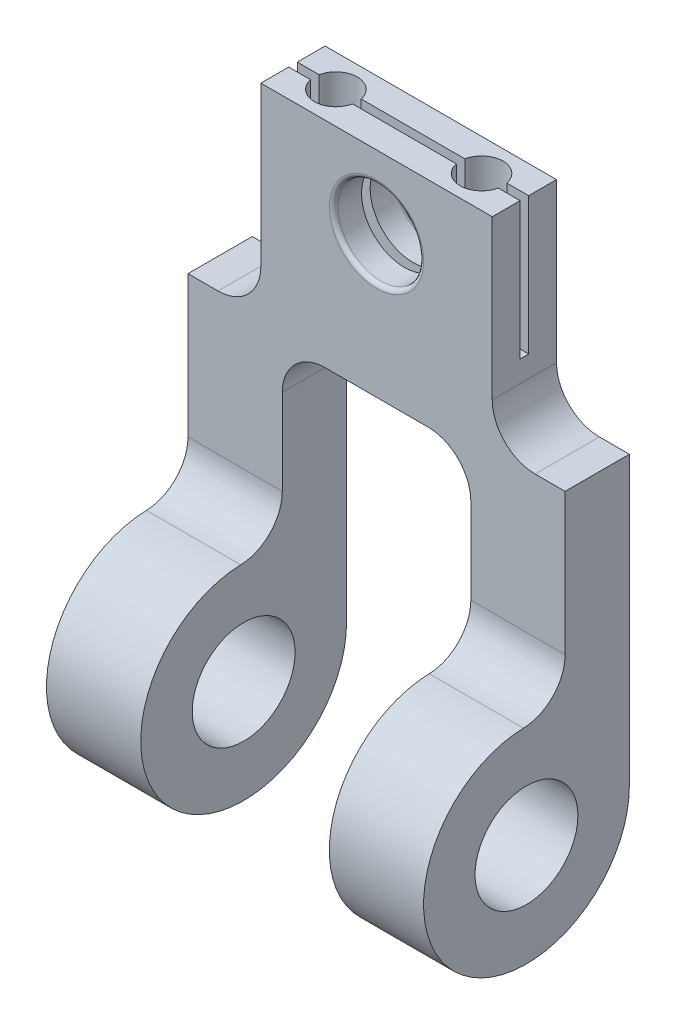
ISO-10303-21;
HEADER;
FILE_DESCRIPTION(('STEP AP214'),'2;1');
FILE_NAME('part.step','',(''),(''),'','','');
FILE_SCHEMA(('AUTOMOTIVE_DESIGN { 1 0 10303 214 1 1 1 1 }'));
ENDSEC;
DATA;
#1=APPLICATION_CONTEXT('core data for automotive mechanical design processes');
#2=APPLICATION_PROTOCOL_DEFINITION('international standard','automotive_design',2000,#1);
#3=PRODUCT_CONTEXT('',#1,'mechanical');
#4=PRODUCT('Part','Part','',(#3));
#5=PRODUCT_RELATED_PRODUCT_CATEGORY('part','',(#4));
#6=PRODUCT_DEFINITION_FORMATION('','',#4);
#7=PRODUCT_DEFINITION_CONTEXT('part definition',#1,'design');
#8=PRODUCT_DEFINITION('design','',#6,#7);
#9=PRODUCT_DEFINITION_SHAPE('','',#8);
#10=(LENGTH_UNIT() NAMED_UNIT(*) SI_UNIT(.MILLI.,.METRE.));
#11=(NAMED_UNIT(*) PLANE_ANGLE_UNIT() SI_UNIT($,.RADIAN.));
#12=(NAMED_UNIT(*) SI_UNIT($,.STERADIAN.) SOLID_ANGLE_UNIT());
#13=UNCERTAINTY_MEASURE_WITH_UNIT(LENGTH_MEASURE(1.E-05),#10,'distance_accuracy_value','');
#14=(GEOMETRIC_REPRESENTATION_CONTEXT(3) GLOBAL_UNCERTAINTY_ASSIGNED_CONTEXT((#13)) GLOBAL_UNIT_ASSIGNED_CONTEXT((#10,
#11,#12)) REPRESENTATION_CONTEXT('',''));
#15=CARTESIAN_POINT('',(0.,0.,0.));
#16=DIRECTION('',(0.,0.,1.));
#17=DIRECTION('',(1.,0.,0.));
#18=AXIS2_PLACEMENT_3D('',#15,#16,#17);
#19=CARTESIAN_POINT('',(44.,114.,-24.01));
#20=DIRECTION('',(0.,-1.,0.));
#21=DIRECTION('',(0.,0.,-1.));
#22=AXIS2_PLACEMENT_3D('',#19,#20,#21);
#23=PLANE('',#22);
#24=CARTESIAN_POINT('',(-17.,114.,-16.51));
#25=DIRECTION('',(0.,1.,0.));
#26=DIRECTION('',(0.,0.,1.));
#27=AXIS2_PLACEMENT_3D('',#24,#25,#26);
#28=CIRCLE('',#27,5.);
#29=CARTESIAN_POINT('',(-21.8989794855664,114.,-15.51));
#30=VERTEX_POINT('',#29);
#31=CARTESIAN_POINT('',(-12.1010205144336,114.,-15.51));
#32=VERTEX_POINT('',#31);
#33=EDGE_CURVE('E499',#30,#32,#28,.T.);
#34=ORIENTED_EDGE('',*,*,#33,.F.);
#35=DIRECTION('',(1.,0.,0.));
#36=VECTOR('',#35,1.);
#37=CARTESIAN_POINT('',(-44.,114.,-15.51));
#38=LINE('',#37,#36);
#39=CARTESIAN_POINT('',(-27.,114.,-15.51));
#40=VERTEX_POINT('',#39);
#41=EDGE_CURVE('E263',#40,#30,#38,.T.);
#42=ORIENTED_EDGE('',*,*,#41,.F.);
#43=DIRECTION('',(0.,0.,1.));
#44=VECTOR('',#43,1.);
#45=CARTESIAN_POINT('',(-27.,114.,-24.01));
#46=LINE('',#45,#44);
#47=CARTESIAN_POINT('',(-27.,114.,-9.01));
#48=VERTEX_POINT('',#47);
#49=EDGE_CURVE('E296',#40,#48,#46,.T.);
#50=ORIENTED_EDGE('',*,*,#49,.T.);
#51=DIRECTION('',(-1.,0.,0.));
#52=VECTOR('',#51,1.);
#53=CARTESIAN_POINT('',(44.,114.,-9.01));
#54=LINE('',#53,#52);
#55=CARTESIAN_POINT('',(27.,114.,-9.01));
#56=VERTEX_POINT('',#55);
#57=EDGE_CURVE('E338',#56,#48,#54,.T.);
#58=ORIENTED_EDGE('',*,*,#57,.F.);
#59=DIRECTION('',(0.,0.,1.));
#60=VECTOR('',#59,1.);
#61=CARTESIAN_POINT('',(27.,114.,-24.01));
#62=LINE('',#61,#60);
#63=CARTESIAN_POINT('',(27.,114.,-15.51));
#64=VERTEX_POINT('',#63);
#65=EDGE_CURVE('E256',#64,#56,#62,.T.);
#66=ORIENTED_EDGE('',*,*,#65,.F.);
#67=CARTESIAN_POINT('',(21.8989794855664,114.,-15.51));
#68=VERTEX_POINT('',#67);
#69=EDGE_CURVE('E252',#68,#64,#38,.T.);
#70=ORIENTED_EDGE('',*,*,#69,.F.);
#71=CARTESIAN_POINT('',(17.,114.,-16.51));
#72=DIRECTION('',(0.,1.,0.));
#73=DIRECTION('',(0.,0.,1.));
#74=AXIS2_PLACEMENT_3D('',#71,#72,#73);
#75=CIRCLE('',#74,5.);
#76=CARTESIAN_POINT('',(12.1010205144336,114.,-15.51));
#77=VERTEX_POINT('',#76);
#78=EDGE_CURVE('E234',#77,#68,#75,.T.);
#79=ORIENTED_EDGE('',*,*,#78,.F.);
#80=EDGE_CURVE('E258',#32,#77,#38,.T.);
#81=ORIENTED_EDGE('',*,*,#80,.F.);
#82=EDGE_LOOP('',(#34,#42,#50,#58,#66,#70,#79,#81));
#83=FACE_BOUND('',#82,.T.);
#84=ADVANCED_FACE('F39',(#83),#23,.F.);
#85=CARTESIAN_POINT('',(-12.1010205144336,114.,-17.51));
#86=VERTEX_POINT('',#85);
#87=CARTESIAN_POINT('',(-21.8989794855664,114.,-17.51));
#88=VERTEX_POINT('',#87);
#89=EDGE_CURVE('E505',#86,#88,#28,.T.);
#90=ORIENTED_EDGE('',*,*,#89,.F.);
#91=DIRECTION('',(1.,0.,0.));
#92=VECTOR('',#91,1.);
#93=CARTESIAN_POINT('',(-44.,114.,-17.51));
#94=LINE('',#93,#92);
#95=CARTESIAN_POINT('',(12.1010205144336,114.,-17.51));
#96=VERTEX_POINT('',#95);
#97=EDGE_CURVE('E261',#86,#96,#94,.T.);
#98=ORIENTED_EDGE('',*,*,#97,.T.);
#99=CARTESIAN_POINT('',(21.8989794855664,114.,-17.51));
#100=VERTEX_POINT('',#99);
#101=EDGE_CURVE('E244',#100,#96,#75,.T.);
#102=ORIENTED_EDGE('',*,*,#101,.F.);
#103=CARTESIAN_POINT('',(27.,114.,-17.51));
#104=VERTEX_POINT('',#103);
#105=EDGE_CURVE('E270',#100,#104,#94,.T.);
#106=ORIENTED_EDGE('',*,*,#105,.T.);
#107=CARTESIAN_POINT('',(27.,114.,-24.01));
#108=VERTEX_POINT('',#107);
#109=EDGE_CURVE('E304',#108,#104,#62,.T.);
#110=ORIENTED_EDGE('',*,*,#109,.F.);
#111=DIRECTION('',(-1.,0.,0.));
#112=VECTOR('',#111,1.);
#113=CARTESIAN_POINT('',(44.,114.,-24.01));
#114=LINE('',#113,#112);
#115=CARTESIAN_POINT('',(-27.,114.,-24.01));
#116=VERTEX_POINT('',#115);
#117=EDGE_CURVE('E347',#108,#116,#114,.T.);
#118=ORIENTED_EDGE('',*,*,#117,.T.);
#119=CARTESIAN_POINT('',(-27.,114.,-17.51));
#120=VERTEX_POINT('',#119);
#121=EDGE_CURVE('E295',#116,#120,#46,.T.);
#122=ORIENTED_EDGE('',*,*,#121,.T.);
#123=EDGE_CURVE('E262',#120,#88,#94,.T.);
#124=ORIENTED_EDGE('',*,*,#123,.T.);
#125=EDGE_LOOP('',(#90,#98,#102,#106,#110,#118,#122,#124));
#126=FACE_BOUND('',#125,.T.);
#127=ADVANCED_FACE('F512',(#126),#23,.F.);
#128=CARTESIAN_POINT('',(-44.,114.,-15.51));
#129=DIRECTION('',(0.,0.,1.));
#130=DIRECTION('',(0.,-1.,0.));
#131=AXIS2_PLACEMENT_3D('',#128,#129,#130);
#132=PLANE('',#131);
#133=CARTESIAN_POINT('',(0.,97.,-15.51));
#134=DIRECTION('',(0.,0.,1.));
#135=DIRECTION('',(0.,-1.,0.));
#136=AXIS2_PLACEMENT_3D('',#133,#134,#135);
#137=CIRCLE('',#136,10.);
#138=CARTESIAN_POINT('',(0.,87.,-15.51));
#139=VERTEX_POINT('',#138);
#140=EDGE_CURVE('E447',#139,#139,#137,.T.);
#141=ORIENTED_EDGE('',*,*,#140,.T.);
#142=EDGE_LOOP('',(#141));
#143=FACE_BOUND('',#142,.T.);
#144=DIRECTION('',(1.,0.,0.));
#145=VECTOR('',#144,1.);
#146=CARTESIAN_POINT('',(-44.,82.,-15.51));
#147=LINE('',#146,#145);
#148=CARTESIAN_POINT('',(-12.1010205144336,82.,-15.51));
#149=VERTEX_POINT('',#148);
#150=CARTESIAN_POINT('',(12.1010205144336,82.,-15.51));
#151=VERTEX_POINT('',#150);
#152=EDGE_CURVE('E476',#149,#151,#147,.T.);
#153=ORIENTED_EDGE('',*,*,#152,.F.);
#154=DIRECTION('',(0.,1.,0.));
#155=VECTOR('',#154,1.);
#156=CARTESIAN_POINT('',(-12.1010205144336,65.,-15.51));
#157=LINE('',#156,#155);
#158=EDGE_CURVE('E450',#149,#32,#157,.T.);
#159=ORIENTED_EDGE('',*,*,#158,.T.);
#160=ORIENTED_EDGE('',*,*,#80,.T.);
#161=DIRECTION('',(0.,1.,0.));
#162=VECTOR('',#161,1.);
#163=CARTESIAN_POINT('',(12.1010205144336,65.,-15.51));
#164=LINE('',#163,#162);
#165=EDGE_CURVE('E239',#77,#151,#164,.F.);
#166=ORIENTED_EDGE('',*,*,#165,.T.);
#167=EDGE_LOOP('',(#153,#159,#160,#166));
#168=FACE_BOUND('',#167,.T.);
#169=ADVANCED_FACE('F519',(#143,#168),#132,.F.);
#170=CARTESIAN_POINT('',(21.8989794855664,82.,-15.51));
#171=VERTEX_POINT('',#170);
#172=CARTESIAN_POINT('',(27.,82.,-15.51));
#173=VERTEX_POINT('',#172);
#174=EDGE_CURVE('E254',#171,#173,#147,.T.);
#175=ORIENTED_EDGE('',*,*,#174,.F.);
#176=DIRECTION('',(0.,1.,0.));
#177=VECTOR('',#176,1.);
#178=CARTESIAN_POINT('',(21.8989794855664,65.,-15.51));
#179=LINE('',#178,#177);
#180=EDGE_CURVE('E240',#171,#68,#179,.T.);
#181=ORIENTED_EDGE('',*,*,#180,.T.);
#182=ORIENTED_EDGE('',*,*,#69,.T.);
#183=DIRECTION('',(0.,1.,0.));
#184=VECTOR('',#183,1.);
#185=CARTESIAN_POINT('',(27.,114.,-15.51));
#186=LINE('',#185,#184);
#187=EDGE_CURVE('E278',#173,#64,#186,.T.);
#188=ORIENTED_EDGE('',*,*,#187,.F.);
#189=EDGE_LOOP('',(#175,#181,#182,#188));
#190=FACE_BOUND('',#189,.T.);
#191=ADVANCED_FACE('F248',(#190),#132,.F.);
#192=CARTESIAN_POINT('',(-44.,114.,-17.51));
#193=DIRECTION('',(0.,0.,-1.));
#194=DIRECTION('',(0.,1.,0.));
#195=AXIS2_PLACEMENT_3D('',#192,#193,#194);
#196=PLANE('',#195);
#197=DIRECTION('',(1.,0.,0.));
#198=VECTOR('',#197,1.);
#199=CARTESIAN_POINT('',(-44.,82.,-17.51));
#200=LINE('',#199,#198);
#201=CARTESIAN_POINT('',(-27.,82.,-17.51));
#202=VERTEX_POINT('',#201);
#203=CARTESIAN_POINT('',(-21.8989794855664,82.,-17.51));
#204=VERTEX_POINT('',#203);
#205=EDGE_CURVE('E468',#202,#204,#200,.T.);
#206=ORIENTED_EDGE('',*,*,#205,.T.);
#207=DIRECTION('',(0.,1.,0.));
#208=VECTOR('',#207,1.);
#209=CARTESIAN_POINT('',(-21.8989794855664,65.,-17.51));
#210=LINE('',#209,#208);
#211=EDGE_CURVE('E65',#204,#88,#210,.T.);
#212=ORIENTED_EDGE('',*,*,#211,.T.);
#213=ORIENTED_EDGE('',*,*,#123,.F.);
#214=DIRECTION('',(0.,1.,0.));
#215=VECTOR('',#214,1.);
#216=CARTESIAN_POINT('',(-27.,114.,-17.51));
#217=LINE('',#216,#215);
#218=EDGE_CURVE('E436',#202,#120,#217,.T.);
#219=ORIENTED_EDGE('',*,*,#218,.F.);
#220=EDGE_LOOP('',(#206,#212,#213,#219));
#221=FACE_BOUND('',#220,.T.);
#222=ADVANCED_FACE('F471',(#221),#196,.F.);
#223=CARTESIAN_POINT('',(0.,97.,-17.51));
#224=DIRECTION('',(0.,0.,-1.));
#225=DIRECTION('',(0.,1.,0.));
#226=AXIS2_PLACEMENT_3D('',#223,#224,#225);
#227=CIRCLE('',#226,10.);
#228=CARTESIAN_POINT('',(0.,107.,-17.51));
#229=VERTEX_POINT('',#228);
#230=EDGE_CURVE('E442',#229,#229,#227,.T.);
#231=ORIENTED_EDGE('',*,*,#230,.T.);
#232=EDGE_LOOP('',(#231));
#233=FACE_BOUND('',#232,.T.);
#234=ORIENTED_EDGE('',*,*,#97,.F.);
#235=DIRECTION('',(0.,1.,0.));
#236=VECTOR('',#235,1.);
#237=CARTESIAN_POINT('',(-12.1010205144336,65.,-17.51));
#238=LINE('',#237,#236);
#239=CARTESIAN_POINT('',(-12.1010205144336,82.,-17.51));
#240=VERTEX_POINT('',#239);
#241=EDGE_CURVE('E487',#86,#240,#238,.F.);
#242=ORIENTED_EDGE('',*,*,#241,.T.);
#243=CARTESIAN_POINT('',(12.1010205144336,82.,-17.51));
#244=VERTEX_POINT('',#243);
#245=EDGE_CURVE('E473',#240,#244,#200,.T.);
#246=ORIENTED_EDGE('',*,*,#245,.T.);
#247=DIRECTION('',(0.,1.,0.));
#248=VECTOR('',#247,1.);
#249=CARTESIAN_POINT('',(12.1010205144336,65.,-17.51));
#250=LINE('',#249,#248);
#251=EDGE_CURVE('E53',#244,#96,#250,.T.);
#252=ORIENTED_EDGE('',*,*,#251,.T.);
#253=EDGE_LOOP('',(#234,#242,#246,#252));
#254=FACE_BOUND('',#253,.T.);
#255=ADVANCED_FACE('F511',(#233,#254),#196,.F.);
#256=CARTESIAN_POINT('',(-44.,82.,-15.51));
#257=DIRECTION('',(0.,-1.,0.));
#258=DIRECTION('',(0.,0.,-1.));
#259=AXIS2_PLACEMENT_3D('',#256,#257,#258);
#260=PLANE('',#259);
#261=ORIENTED_EDGE('',*,*,#245,.F.);
#262=CARTESIAN_POINT('',(-17.,82.,-16.51));
#263=DIRECTION('',(0.,-1.,0.));
#264=DIRECTION('',(0.,0.,-1.));
#265=AXIS2_PLACEMENT_3D('',#262,#263,#264);
#266=CIRCLE('',#265,5.);
#267=EDGE_CURVE('E11',#240,#149,#266,.T.);
#268=ORIENTED_EDGE('',*,*,#267,.T.);
#269=ORIENTED_EDGE('',*,*,#152,.T.);
#270=CARTESIAN_POINT('',(17.,82.,-16.51));
#271=DIRECTION('',(0.,-1.,0.));
#272=DIRECTION('',(0.,0.,-1.));
#273=AXIS2_PLACEMENT_3D('',#270,#271,#272);
#274=CIRCLE('',#273,5.);
#275=EDGE_CURVE('E458',#151,#244,#274,.T.);
#276=ORIENTED_EDGE('',*,*,#275,.T.);
#277=EDGE_LOOP('',(#261,#268,#269,#276));
#278=FACE_BOUND('',#277,.T.);
#279=ADVANCED_FACE('F513',(#278),#260,.F.);
#280=CARTESIAN_POINT('',(21.8989794855664,82.,-17.51));
#281=VERTEX_POINT('',#280);
#282=CARTESIAN_POINT('',(27.,82.,-17.51));
#283=VERTEX_POINT('',#282);
#284=EDGE_CURVE('E477',#281,#283,#200,.T.);
#285=ORIENTED_EDGE('',*,*,#284,.F.);
#286=EDGE_CURVE('E459',#281,#171,#274,.T.);
#287=ORIENTED_EDGE('',*,*,#286,.T.);
#288=ORIENTED_EDGE('',*,*,#174,.T.);
#289=DIRECTION('',(0.,0.,1.));
#290=VECTOR('',#289,1.);
#291=CARTESIAN_POINT('',(27.,82.,-24.01));
#292=LINE('',#291,#290);
#293=EDGE_CURVE('E269',#283,#173,#292,.T.);
#294=ORIENTED_EDGE('',*,*,#293,.F.);
#295=EDGE_LOOP('',(#285,#287,#288,#294));
#296=FACE_BOUND('',#295,.T.);
#297=ADVANCED_FACE('F600',(#296),#260,.F.);
#298=CARTESIAN_POINT('',(44.,0.,0.));
#299=DIRECTION('',(1.,0.,0.));
#300=DIRECTION('',(0.,0.,-1.));
#301=AXIS2_PLACEMENT_3D('',#298,#299,#300);
#302=PLANE('',#301);
#303=CARTESIAN_POINT('',(44.,0.,0.));
#304=DIRECTION('',(1.,0.,0.));
#305=DIRECTION('',(0.,0.,-1.));
#306=AXIS2_PLACEMENT_3D('',#303,#304,#305);
#307=CIRCLE('',#306,12.);
#308=CARTESIAN_POINT('',(44.,0.,-12.));
#309=VERTEX_POINT('',#308);
#310=EDGE_CURVE('E352',#309,#309,#307,.T.);
#311=ORIENTED_EDGE('',*,*,#310,.F.);
#312=EDGE_LOOP('',(#311));
#313=FACE_BOUND('',#312,.T.);
#314=DIRECTION('',(0.,1.,0.));
#315=VECTOR('',#314,1.);
#316=CARTESIAN_POINT('',(44.,0.,-24.01));
#317=LINE('',#316,#315);
#318=CARTESIAN_POINT('',(44.,0.,-24.01));
#319=VERTEX_POINT('',#318);
#320=CARTESIAN_POINT('',(44.,67.,-24.01));
#321=VERTEX_POINT('',#320);
#322=EDGE_CURVE('E332',#319,#321,#317,.T.);
#323=ORIENTED_EDGE('',*,*,#322,.T.);
#324=DIRECTION('',(0.,0.,1.));
#325=VECTOR('',#324,1.);
#326=CARTESIAN_POINT('',(44.,67.,-24.01));
#327=LINE('',#326,#325);
#328=CARTESIAN_POINT('',(44.,67.,-9.01));
#329=VERTEX_POINT('',#328);
#330=EDGE_CURVE('E301',#321,#329,#327,.T.);
#331=ORIENTED_EDGE('',*,*,#330,.T.);
#332=DIRECTION('',(0.,-1.,0.));
#333=VECTOR('',#332,1.);
#334=CARTESIAN_POINT('',(44.,114.,-9.01));
#335=LINE('',#334,#333);
#336=CARTESIAN_POINT('',(44.,33.9955879490266,-9.01000000000001));
#337=VERTEX_POINT('',#336);
#338=EDGE_CURVE('E340',#329,#337,#335,.T.);
#339=ORIENTED_EDGE('',*,*,#338,.T.);
#340=CARTESIAN_POINT('',(44.,33.9955879490266,0.989999999999993));
#341=DIRECTION('',(1.,0.,0.));
#342=DIRECTION('',(0.,0.,-1.));
#343=AXIS2_PLACEMENT_3D('',#340,#341,#342);
#344=CIRCLE('',#343,10.);
#345=CARTESIAN_POINT('',(44.,23.9998255411975,0.698909144369299));
#346=VERTEX_POINT('',#345);
#347=EDGE_CURVE('E374',#337,#346,#344,.F.);
#348=ORIENTED_EDGE('',*,*,#347,.T.);
#349=CARTESIAN_POINT('',(44.,0.,0.));
#350=DIRECTION('',(1.,0.,0.));
#351=DIRECTION('',(0.,0.,-1.));
#352=AXIS2_PLACEMENT_3D('',#349,#350,#351);
#353=CIRCLE('',#352,24.01);
#354=EDGE_CURVE('E359',#346,#319,#353,.T.);
#355=ORIENTED_EDGE('',*,*,#354,.T.);
#356=EDGE_LOOP('',(#323,#331,#339,#348,#355));
#357=FACE_BOUND('',#356,.T.);
#358=ADVANCED_FACE('F543',(#313,#357),#302,.T.);
#359=CARTESIAN_POINT('',(-44.,0.,0.));
#360=DIRECTION('',(1.,0.,0.));
#361=DIRECTION('',(0.,0.,-1.));
#362=AXIS2_PLACEMENT_3D('',#359,#360,#361);
#363=PLANE('',#362);
#364=CARTESIAN_POINT('',(-44.,0.,0.));
#365=DIRECTION('',(1.,0.,0.));
#366=DIRECTION('',(0.,0.,-1.));
#367=AXIS2_PLACEMENT_3D('',#364,#365,#366);
#368=CIRCLE('',#367,12.);
#369=CARTESIAN_POINT('',(-44.,0.,-12.));
#370=VERTEX_POINT('',#369);
#371=EDGE_CURVE('E351',#370,#370,#368,.T.);
#372=ORIENTED_EDGE('',*,*,#371,.T.);
#373=EDGE_LOOP('',(#372));
#374=FACE_BOUND('',#373,.T.);
#375=DIRECTION('',(0.,0.,1.));
#376=VECTOR('',#375,1.);
#377=CARTESIAN_POINT('',(-44.,67.,-24.01));
#378=LINE('',#377,#376);
#379=CARTESIAN_POINT('',(-44.,67.,-24.01));
#380=VERTEX_POINT('',#379);
#381=CARTESIAN_POINT('',(-44.,67.,-9.01));
#382=VERTEX_POINT('',#381);
#383=EDGE_CURVE('E291',#380,#382,#378,.T.);
#384=ORIENTED_EDGE('',*,*,#383,.F.);
#385=DIRECTION('',(0.,1.,0.));
#386=VECTOR('',#385,1.);
#387=CARTESIAN_POINT('',(-44.,0.,-24.01));
#388=LINE('',#387,#386);
#389=CARTESIAN_POINT('',(-44.,0.,-24.01));
#390=VERTEX_POINT('',#389);
#391=EDGE_CURVE('E331',#390,#380,#388,.T.);
#392=ORIENTED_EDGE('',*,*,#391,.F.);
#393=CARTESIAN_POINT('',(-44.,0.,0.));
#394=DIRECTION('',(1.,0.,0.));
#395=DIRECTION('',(0.,0.,-1.));
#396=AXIS2_PLACEMENT_3D('',#393,#394,#395);
#397=CIRCLE('',#396,24.01);
#398=CARTESIAN_POINT('',(-44.,23.9998255411975,0.698909144369299));
#399=VERTEX_POINT('',#398);
#400=EDGE_CURVE('E357',#399,#390,#397,.T.);
#401=ORIENTED_EDGE('',*,*,#400,.F.);
#402=CARTESIAN_POINT('',(-44.,33.9955879490266,0.989999999999993));
#403=DIRECTION('',(1.,0.,0.));
#404=DIRECTION('',(0.,0.,-1.));
#405=AXIS2_PLACEMENT_3D('',#402,#403,#404);
#406=CIRCLE('',#405,10.);
#407=CARTESIAN_POINT('',(-44.,33.9955879490266,-9.01000000000001));
#408=VERTEX_POINT('',#407);
#409=EDGE_CURVE('E375',#399,#408,#406,.T.);
#410=ORIENTED_EDGE('',*,*,#409,.T.);
#411=DIRECTION('',(0.,-1.,0.));
#412=VECTOR('',#411,1.);
#413=CARTESIAN_POINT('',(-44.,114.,-9.01));
#414=LINE('',#413,#412);
#415=EDGE_CURVE('E336',#382,#408,#414,.T.);
#416=ORIENTED_EDGE('',*,*,#415,.F.);
#417=EDGE_LOOP('',(#384,#392,#401,#410,#416));
#418=FACE_BOUND('',#417,.T.);
#419=ADVANCED_FACE('F585',(#374,#418),#363,.F.);
#420=CARTESIAN_POINT('',(44.,0.,0.));
#421=DIRECTION('',(-1.,0.,0.));
#422=DIRECTION('',(0.,0.,1.));
#423=AXIS2_PLACEMENT_3D('',#420,#421,#422);
#424=CYLINDRICAL_SURFACE('',#423,24.01);
#425=CARTESIAN_POINT('',(-22.,0.,0.));
#426=DIRECTION('',(-1.,0.,0.));
#427=DIRECTION('',(0.,-1.,0.));
#428=AXIS2_PLACEMENT_3D('',#425,#426,#427);
#429=CIRCLE('',#428,24.01);
#430=CARTESIAN_POINT('',(-22.,0.,-24.01));
#431=VERTEX_POINT('',#430);
#432=CARTESIAN_POINT('',(-22.,23.9998255411975,0.698909144369299));
#433=VERTEX_POINT('',#432);
#434=EDGE_CURVE('E328',#431,#433,#429,.T.);
#435=ORIENTED_EDGE('',*,*,#434,.T.);
#436=DIRECTION('',(-1.,0.,0.));
#437=VECTOR('',#436,1.);
#438=CARTESIAN_POINT('',(44.,23.9998255411975,0.698909144369299));
#439=LINE('',#438,#437);
#440=EDGE_CURVE('E365',#433,#399,#439,.T.);
#441=ORIENTED_EDGE('',*,*,#440,.T.);
#442=ORIENTED_EDGE('',*,*,#400,.T.);
#443=DIRECTION('',(-1.,0.,0.));
#444=VECTOR('',#443,1.);
#445=CARTESIAN_POINT('',(44.,0.,-24.01));
#446=LINE('',#445,#444);
#447=EDGE_CURVE('E349',#431,#390,#446,.T.);
#448=ORIENTED_EDGE('',*,*,#447,.F.);
#449=EDGE_LOOP('',(#435,#441,#442,#448));
#450=FACE_BOUND('',#449,.T.);
#451=ADVANCED_FACE('F580',(#450),#424,.T.);
#452=CARTESIAN_POINT('',(44.,0.,0.));
#453=DIRECTION('',(-1.,0.,0.));
#454=DIRECTION('',(0.,0.,1.));
#455=AXIS2_PLACEMENT_3D('',#452,#453,#454);
#456=CYLINDRICAL_SURFACE('',#455,12.);
#457=CARTESIAN_POINT('',(-22.,0.,0.));
#458=DIRECTION('',(-1.,0.,0.));
#459=DIRECTION('',(0.,-1.,0.));
#460=AXIS2_PLACEMENT_3D('',#457,#458,#459);
#461=CIRCLE('',#460,12.);
#462=CARTESIAN_POINT('',(-22.,-12.,0.));
#463=VERTEX_POINT('',#462);
#464=EDGE_CURVE('E326',#463,#463,#461,.T.);
#465=ORIENTED_EDGE('',*,*,#464,.F.);
#466=EDGE_LOOP('',(#465));
#467=FACE_BOUND('',#466,.T.);
#468=ORIENTED_EDGE('',*,*,#371,.F.);
#469=EDGE_LOOP('',(#468));
#470=FACE_BOUND('',#469,.T.);
#471=ADVANCED_FACE('F626',(#467,#470),#456,.F.);
#472=CARTESIAN_POINT('',(44.,33.9955879490266,0.989999999999993));
#473=DIRECTION('',(-1.,0.,0.));
#474=DIRECTION('',(0.,0.,1.));
#475=AXIS2_PLACEMENT_3D('',#472,#473,#474);
#476=CYLINDRICAL_SURFACE('',#475,10.);
#477=ORIENTED_EDGE('',*,*,#440,.F.);
#478=CARTESIAN_POINT('',(-22.,33.9955879490266,0.989999999999993));
#479=DIRECTION('',(-1.,0.,0.));
#480=DIRECTION('',(0.,-1.,0.));
#481=AXIS2_PLACEMENT_3D('',#478,#479,#480);
#482=CIRCLE('',#481,10.);
#483=CARTESIAN_POINT('',(-22.,33.9955879490266,-9.01000000000001));
#484=VERTEX_POINT('',#483);
#485=EDGE_CURVE('E379',#433,#484,#482,.F.);
#486=ORIENTED_EDGE('',*,*,#485,.T.);
#487=DIRECTION('',(1.,0.,0.));
#488=VECTOR('',#487,1.);
#489=CARTESIAN_POINT('',(44.,33.9955879490266,-9.01000000000001));
#490=LINE('',#489,#488);
#491=EDGE_CURVE('E367',#408,#484,#490,.T.);
#492=ORIENTED_EDGE('',*,*,#491,.F.);
#493=ORIENTED_EDGE('',*,*,#409,.F.);
#494=EDGE_LOOP('',(#477,#486,#492,#493));
#495=FACE_BOUND('',#494,.T.);
#496=ADVANCED_FACE('F633',(#495),#476,.F.);
#497=CARTESIAN_POINT('',(22.,23.9998255411975,0.698909144369299));
#498=VERTEX_POINT('',#497);
#499=EDGE_CURVE('E362',#346,#498,#439,.T.);
#500=ORIENTED_EDGE('',*,*,#499,.T.);
#501=CARTESIAN_POINT('',(22.,0.,0.));
#502=DIRECTION('',(1.,0.,0.));
#503=DIRECTION('',(0.,1.,0.));
#504=AXIS2_PLACEMENT_3D('',#501,#502,#503);
#505=CIRCLE('',#504,24.01);
#506=CARTESIAN_POINT('',(22.,0.,-24.01));
#507=VERTEX_POINT('',#506);
#508=EDGE_CURVE('E318',#498,#507,#505,.T.);
#509=ORIENTED_EDGE('',*,*,#508,.T.);
#510=EDGE_CURVE('E346',#319,#507,#446,.T.);
#511=ORIENTED_EDGE('',*,*,#510,.F.);
#512=ORIENTED_EDGE('',*,*,#354,.F.);
#513=EDGE_LOOP('',(#500,#509,#511,#512));
#514=FACE_BOUND('',#513,.T.);
#515=ADVANCED_FACE('F550',(#514),#424,.T.);
#516=CARTESIAN_POINT('',(22.,0.,0.));
#517=DIRECTION('',(1.,0.,0.));
#518=DIRECTION('',(0.,1.,0.));
#519=AXIS2_PLACEMENT_3D('',#516,#517,#518);
#520=CIRCLE('',#519,12.);
#521=CARTESIAN_POINT('',(22.,12.,0.));
#522=VERTEX_POINT('',#521);
#523=EDGE_CURVE('E325',#522,#522,#520,.T.);
#524=ORIENTED_EDGE('',*,*,#523,.F.);
#525=EDGE_LOOP('',(#524));
#526=FACE_BOUND('',#525,.T.);
#527=ORIENTED_EDGE('',*,*,#310,.T.);
#528=EDGE_LOOP('',(#527));
#529=FACE_BOUND('',#528,.T.);
#530=ADVANCED_FACE('F625',(#526,#529),#456,.F.);
#531=CARTESIAN_POINT('',(44.,0.,-24.01));
#532=DIRECTION('',(0.,0.,1.));
#533=DIRECTION('',(0.,-1.,0.));
#534=AXIS2_PLACEMENT_3D('',#531,#532,#533);
#535=PLANE('',#534);
#536=CARTESIAN_POINT('',(0.,97.,-24.01));
#537=DIRECTION('',(0.,0.,1.));
#538=DIRECTION('',(0.,-1.,0.));
#539=AXIS2_PLACEMENT_3D('',#536,#537,#538);
#540=CIRCLE('',#539,11.);
#541=CARTESIAN_POINT('',(0.,86.,-24.01));
#542=VERTEX_POINT('',#541);
#543=EDGE_CURVE('E445',#542,#542,#540,.T.);
#544=ORIENTED_EDGE('',*,*,#543,.T.);
#545=EDGE_LOOP('',(#544));
#546=FACE_BOUND('',#545,.T.);
#547=DIRECTION('',(1.,0.,0.));
#548=VECTOR('',#547,1.);
#549=CARTESIAN_POINT('',(-44.,67.,-24.01));
#550=LINE('',#549,#548);
#551=CARTESIAN_POINT('',(-37.,67.,-24.01));
#552=VERTEX_POINT('',#551);
#553=EDGE_CURVE('E290',#380,#552,#550,.T.);
#554=ORIENTED_EDGE('',*,*,#553,.T.);
#555=CARTESIAN_POINT('',(-37.,77.,-24.01));
#556=DIRECTION('',(0.,0.,1.));
#557=DIRECTION('',(0.,-1.,0.));
#558=AXIS2_PLACEMENT_3D('',#555,#556,#557);
#559=CIRCLE('',#558,10.);
#560=CARTESIAN_POINT('',(-27.,77.,-24.01));
#561=VERTEX_POINT('',#560);
#562=EDGE_CURVE('E430',#552,#561,#559,.T.);
#563=ORIENTED_EDGE('',*,*,#562,.T.);
#564=DIRECTION('',(0.,1.,0.));
#565=VECTOR('',#564,1.);
#566=CARTESIAN_POINT('',(-27.,114.,-24.01));
#567=LINE('',#566,#565);
#568=EDGE_CURVE('E289',#561,#116,#567,.T.);
#569=ORIENTED_EDGE('',*,*,#568,.T.);
#570=ORIENTED_EDGE('',*,*,#117,.F.);
#571=DIRECTION('',(0.,-1.,0.));
#572=VECTOR('',#571,1.);
#573=CARTESIAN_POINT('',(27.,114.,-24.01));
#574=LINE('',#573,#572);
#575=CARTESIAN_POINT('',(27.,77.,-24.01));
#576=VERTEX_POINT('',#575);
#577=EDGE_CURVE('E302',#108,#576,#574,.T.);
#578=ORIENTED_EDGE('',*,*,#577,.T.);
#579=CARTESIAN_POINT('',(37.,77.,-24.01));
#580=DIRECTION('',(0.,0.,1.));
#581=DIRECTION('',(0.,-1.,0.));
#582=AXIS2_PLACEMENT_3D('',#579,#580,#581);
#583=CIRCLE('',#582,10.);
#584=CARTESIAN_POINT('',(37.,67.,-24.01));
#585=VERTEX_POINT('',#584);
#586=EDGE_CURVE('E431',#576,#585,#583,.T.);
#587=ORIENTED_EDGE('',*,*,#586,.T.);
#588=DIRECTION('',(1.,0.,0.));
#589=VECTOR('',#588,1.);
#590=CARTESIAN_POINT('',(27.,67.,-24.01));
#591=LINE('',#590,#589);
#592=EDGE_CURVE('E293',#585,#321,#591,.T.);
#593=ORIENTED_EDGE('',*,*,#592,.T.);
#594=ORIENTED_EDGE('',*,*,#322,.F.);
#595=ORIENTED_EDGE('',*,*,#510,.T.);
#596=DIRECTION('',(0.,1.,0.));
#597=VECTOR('',#596,1.);
#598=CARTESIAN_POINT('',(22.,64.,-24.01));
#599=LINE('',#598,#597);
#600=CARTESIAN_POINT('',(22.,54.,-24.01));
#601=VERTEX_POINT('',#600);
#602=EDGE_CURVE('E315',#507,#601,#599,.T.);
#603=ORIENTED_EDGE('',*,*,#602,.T.);
#604=CARTESIAN_POINT('',(12.,54.,-24.01));
#605=DIRECTION('',(0.,0.,1.));
#606=DIRECTION('',(0.,-1.,0.));
#607=AXIS2_PLACEMENT_3D('',#604,#605,#606);
#608=CIRCLE('',#607,10.);
#609=CARTESIAN_POINT('',(12.,64.,-24.01));
#610=VERTEX_POINT('',#609);
#611=EDGE_CURVE('E417',#601,#610,#608,.T.);
#612=ORIENTED_EDGE('',*,*,#611,.T.);
#613=DIRECTION('',(-1.,0.,0.));
#614=VECTOR('',#613,1.);
#615=CARTESIAN_POINT('',(-22.,64.,-24.01));
#616=LINE('',#615,#614);
#617=CARTESIAN_POINT('',(-12.,64.,-24.01));
#618=VERTEX_POINT('',#617);
#619=EDGE_CURVE('E314',#610,#618,#616,.T.);
#620=ORIENTED_EDGE('',*,*,#619,.T.);
#621=CARTESIAN_POINT('',(-12.,54.,-24.01));
#622=DIRECTION('',(0.,0.,1.));
#623=DIRECTION('',(0.,-1.,0.));
#624=AXIS2_PLACEMENT_3D('',#621,#622,#623);
#625=CIRCLE('',#624,10.);
#626=CARTESIAN_POINT('',(-22.,54.,-24.01));
#627=VERTEX_POINT('',#626);
#628=EDGE_CURVE('E421',#618,#627,#625,.T.);
#629=ORIENTED_EDGE('',*,*,#628,.T.);
#630=DIRECTION('',(0.,-1.,0.));
#631=VECTOR('',#630,1.);
#632=CARTESIAN_POINT('',(-22.,64.,-24.01));
#633=LINE('',#632,#631);
#634=EDGE_CURVE('E300',#627,#431,#633,.T.);
#635=ORIENTED_EDGE('',*,*,#634,.T.);
#636=ORIENTED_EDGE('',*,*,#447,.T.);
#637=ORIENTED_EDGE('',*,*,#391,.T.);
#638=EDGE_LOOP('',(#554,#563,#569,#570,#578,#587,#593,#594,#595,#603,#612,#620,#629,#635,#636,#637));
#639=FACE_BOUND('',#638,.T.);
#640=ADVANCED_FACE('F533',(#546,#639),#535,.F.);
#641=CARTESIAN_POINT('',(44.,114.,-9.01));
#642=DIRECTION('',(0.,0.,-1.));
#643=DIRECTION('',(0.,1.,0.));
#644=AXIS2_PLACEMENT_3D('',#641,#642,#643);
#645=PLANE('',#644);
#646=CARTESIAN_POINT('',(0.,97.,-9.01));
#647=DIRECTION('',(0.,0.,-1.));
#648=DIRECTION('',(0.,1.,0.));
#649=AXIS2_PLACEMENT_3D('',#646,#647,#648);
#650=CIRCLE('',#649,11.);
#651=CARTESIAN_POINT('',(0.,108.,-9.01));
#652=VERTEX_POINT('',#651);
#653=EDGE_CURVE('E454',#652,#652,#650,.T.);
#654=ORIENTED_EDGE('',*,*,#653,.T.);
#655=EDGE_LOOP('',(#654));
#656=FACE_BOUND('',#655,.T.);
#657=ORIENTED_EDGE('',*,*,#57,.T.);
#658=DIRECTION('',(0.,-1.,0.));
#659=VECTOR('',#658,1.);
#660=CARTESIAN_POINT('',(-27.,114.,-9.01));
#661=LINE('',#660,#659);
#662=CARTESIAN_POINT('',(-27.,77.,-9.01));
#663=VERTEX_POINT('',#662);
#664=EDGE_CURVE('E394',#48,#663,#661,.T.);
#665=ORIENTED_EDGE('',*,*,#664,.T.);
#666=CARTESIAN_POINT('',(-37.,77.,-9.01));
#667=DIRECTION('',(0.,0.,-1.));
#668=DIRECTION('',(0.,1.,0.));
#669=AXIS2_PLACEMENT_3D('',#666,#667,#668);
#670=CIRCLE('',#669,10.);
#671=CARTESIAN_POINT('',(-37.,67.,-9.01));
#672=VERTEX_POINT('',#671);
#673=EDGE_CURVE('E424',#663,#672,#670,.T.);
#674=ORIENTED_EDGE('',*,*,#673,.T.);
#675=DIRECTION('',(-1.,0.,0.));
#676=VECTOR('',#675,1.);
#677=CARTESIAN_POINT('',(44.,67.,-9.01));
#678=LINE('',#677,#676);
#679=EDGE_CURVE('E395',#672,#382,#678,.T.);
#680=ORIENTED_EDGE('',*,*,#679,.T.);
#681=ORIENTED_EDGE('',*,*,#415,.T.);
#682=ORIENTED_EDGE('',*,*,#491,.T.);
#683=DIRECTION('',(0.,1.,0.));
#684=VECTOR('',#683,1.);
#685=CARTESIAN_POINT('',(-22.,114.,-9.01));
#686=LINE('',#685,#684);
#687=CARTESIAN_POINT('',(-22.,54.,-9.01000000000001));
#688=VERTEX_POINT('',#687);
#689=EDGE_CURVE('E323',#484,#688,#686,.T.);
#690=ORIENTED_EDGE('',*,*,#689,.T.);
#691=CARTESIAN_POINT('',(-12.,54.,-9.01000000000001));
#692=DIRECTION('',(0.,0.,-1.));
#693=DIRECTION('',(0.,1.,0.));
#694=AXIS2_PLACEMENT_3D('',#691,#692,#693);
#695=CIRCLE('',#694,10.);
#696=CARTESIAN_POINT('',(-12.,64.,-9.01));
#697=VERTEX_POINT('',#696);
#698=EDGE_CURVE('E423',#688,#697,#695,.T.);
#699=ORIENTED_EDGE('',*,*,#698,.T.);
#700=DIRECTION('',(1.,0.,0.));
#701=VECTOR('',#700,1.);
#702=CARTESIAN_POINT('',(44.,64.,-9.01));
#703=LINE('',#702,#701);
#704=CARTESIAN_POINT('',(12.,64.,-9.01));
#705=VERTEX_POINT('',#704);
#706=EDGE_CURVE('E384',#697,#705,#703,.T.);
#707=ORIENTED_EDGE('',*,*,#706,.T.);
#708=CARTESIAN_POINT('',(12.,54.,-9.01000000000001));
#709=DIRECTION('',(0.,0.,-1.));
#710=DIRECTION('',(0.,1.,0.));
#711=AXIS2_PLACEMENT_3D('',#708,#709,#710);
#712=CIRCLE('',#711,10.);
#713=CARTESIAN_POINT('',(22.,54.,-9.01000000000001));
#714=VERTEX_POINT('',#713);
#715=EDGE_CURVE('E420',#705,#714,#712,.T.);
#716=ORIENTED_EDGE('',*,*,#715,.T.);
#717=DIRECTION('',(0.,-1.,0.));
#718=VECTOR('',#717,1.);
#719=CARTESIAN_POINT('',(22.,114.,-9.01));
#720=LINE('',#719,#718);
#721=CARTESIAN_POINT('',(22.,33.9955879490266,-9.01000000000001));
#722=VERTEX_POINT('',#721);
#723=EDGE_CURVE('E319',#714,#722,#720,.T.);
#724=ORIENTED_EDGE('',*,*,#723,.T.);
#725=EDGE_CURVE('E368',#722,#337,#490,.T.);
#726=ORIENTED_EDGE('',*,*,#725,.T.);
#727=ORIENTED_EDGE('',*,*,#338,.F.);
#728=DIRECTION('',(-1.,0.,0.));
#729=VECTOR('',#728,1.);
#730=CARTESIAN_POINT('',(44.,67.,-9.01));
#731=LINE('',#730,#729);
#732=CARTESIAN_POINT('',(37.,67.,-9.01));
#733=VERTEX_POINT('',#732);
#734=EDGE_CURVE('E386',#329,#733,#731,.T.);
#735=ORIENTED_EDGE('',*,*,#734,.T.);
#736=CARTESIAN_POINT('',(37.,77.,-9.01));
#737=DIRECTION('',(0.,0.,-1.));
#738=DIRECTION('',(0.,1.,0.));
#739=AXIS2_PLACEMENT_3D('',#736,#737,#738);
#740=CIRCLE('',#739,10.);
#741=CARTESIAN_POINT('',(27.,77.,-9.01));
#742=VERTEX_POINT('',#741);
#743=EDGE_CURVE('E429',#733,#742,#740,.T.);
#744=ORIENTED_EDGE('',*,*,#743,.T.);
#745=DIRECTION('',(0.,1.,0.));
#746=VECTOR('',#745,1.);
#747=CARTESIAN_POINT('',(27.,114.,-9.01));
#748=LINE('',#747,#746);
#749=EDGE_CURVE('E387',#742,#56,#748,.T.);
#750=ORIENTED_EDGE('',*,*,#749,.T.);
#751=EDGE_LOOP('',(#657,#665,#674,#680,#681,#682,#690,#699,#707,#716,#724,#726,#727,#735,#744,#750));
#752=FACE_BOUND('',#751,.T.);
#753=ADVANCED_FACE('F521',(#656,#752),#645,.F.);
#754=ORIENTED_EDGE('',*,*,#725,.F.);
#755=CARTESIAN_POINT('',(22.,33.9955879490266,0.989999999999993));
#756=DIRECTION('',(1.,0.,0.));
#757=DIRECTION('',(0.,1.,0.));
#758=AXIS2_PLACEMENT_3D('',#755,#756,#757);
#759=CIRCLE('',#758,10.);
#760=EDGE_CURVE('E380',#722,#498,#759,.F.);
#761=ORIENTED_EDGE('',*,*,#760,.T.);
#762=ORIENTED_EDGE('',*,*,#499,.F.);
#763=ORIENTED_EDGE('',*,*,#347,.F.);
#764=EDGE_LOOP('',(#754,#761,#762,#763));
#765=FACE_BOUND('',#764,.T.);
#766=ADVANCED_FACE('F632',(#765),#476,.F.);
#767=CARTESIAN_POINT('',(-22.,64.,-24.01));
#768=DIRECTION('',(0.,1.,0.));
#769=DIRECTION('',(0.,0.,1.));
#770=AXIS2_PLACEMENT_3D('',#767,#768,#769);
#771=PLANE('',#770);
#772=ORIENTED_EDGE('',*,*,#619,.F.);
#773=DIRECTION('',(0.,0.,1.));
#774=VECTOR('',#773,1.);
#775=CARTESIAN_POINT('',(12.,64.,-9.01));
#776=LINE('',#775,#774);
#777=EDGE_CURVE('E397',#610,#705,#776,.T.);
#778=ORIENTED_EDGE('',*,*,#777,.T.);
#779=ORIENTED_EDGE('',*,*,#706,.F.);
#780=DIRECTION('',(0.,0.,1.));
#781=VECTOR('',#780,1.);
#782=CARTESIAN_POINT('',(-12.,64.,-24.01));
#783=LINE('',#782,#781);
#784=EDGE_CURVE('E400',#697,#618,#783,.F.);
#785=ORIENTED_EDGE('',*,*,#784,.T.);
#786=EDGE_LOOP('',(#772,#778,#779,#785));
#787=FACE_BOUND('',#786,.T.);
#788=ADVANCED_FACE('F565',(#787),#771,.F.);
#789=CARTESIAN_POINT('',(-22.,64.,-24.01));
#790=DIRECTION('',(-1.,0.,0.));
#791=DIRECTION('',(0.,-1.,0.));
#792=AXIS2_PLACEMENT_3D('',#789,#790,#791);
#793=PLANE('',#792);
#794=ORIENTED_EDGE('',*,*,#464,.T.);
#795=EDGE_LOOP('',(#794));
#796=FACE_BOUND('',#795,.T.);
#797=ORIENTED_EDGE('',*,*,#634,.F.);
#798=DIRECTION('',(0.,0.,1.));
#799=VECTOR('',#798,1.);
#800=CARTESIAN_POINT('',(-22.,54.,-9.01));
#801=LINE('',#800,#799);
#802=EDGE_CURVE('E404',#627,#688,#801,.T.);
#803=ORIENTED_EDGE('',*,*,#802,.T.);
#804=ORIENTED_EDGE('',*,*,#689,.F.);
#805=ORIENTED_EDGE('',*,*,#485,.F.);
#806=ORIENTED_EDGE('',*,*,#434,.F.);
#807=EDGE_LOOP('',(#797,#803,#804,#805,#806));
#808=FACE_BOUND('',#807,.T.);
#809=ADVANCED_FACE('F569',(#796,#808),#793,.F.);
#810=CARTESIAN_POINT('',(22.,64.,-24.01));
#811=DIRECTION('',(1.,0.,0.));
#812=DIRECTION('',(0.,1.,0.));
#813=AXIS2_PLACEMENT_3D('',#810,#811,#812);
#814=PLANE('',#813);
#815=ORIENTED_EDGE('',*,*,#523,.T.);
#816=EDGE_LOOP('',(#815));
#817=FACE_BOUND('',#816,.T.);
#818=ORIENTED_EDGE('',*,*,#723,.F.);
#819=DIRECTION('',(0.,0.,1.));
#820=VECTOR('',#819,1.);
#821=CARTESIAN_POINT('',(22.,54.,-24.01));
#822=LINE('',#821,#820);
#823=EDGE_CURVE('E405',#714,#601,#822,.F.);
#824=ORIENTED_EDGE('',*,*,#823,.T.);
#825=ORIENTED_EDGE('',*,*,#602,.F.);
#826=ORIENTED_EDGE('',*,*,#508,.F.);
#827=ORIENTED_EDGE('',*,*,#760,.F.);
#828=EDGE_LOOP('',(#818,#824,#825,#826,#827));
#829=FACE_BOUND('',#828,.T.);
#830=ADVANCED_FACE('F551',(#817,#829),#814,.F.);
#831=CARTESIAN_POINT('',(27.,67.,-24.01));
#832=DIRECTION('',(0.,-1.,0.));
#833=DIRECTION('',(0.,0.,-1.));
#834=AXIS2_PLACEMENT_3D('',#831,#832,#833);
#835=PLANE('',#834);
#836=ORIENTED_EDGE('',*,*,#592,.F.);
#837=DIRECTION('',(0.,0.,1.));
#838=VECTOR('',#837,1.);
#839=CARTESIAN_POINT('',(37.,67.,-9.01));
#840=LINE('',#839,#838);
#841=EDGE_CURVE('E415',#585,#733,#840,.T.);
#842=ORIENTED_EDGE('',*,*,#841,.T.);
#843=ORIENTED_EDGE('',*,*,#734,.F.);
#844=ORIENTED_EDGE('',*,*,#330,.F.);
#845=EDGE_LOOP('',(#836,#842,#843,#844));
#846=FACE_BOUND('',#845,.T.);
#847=ADVANCED_FACE('F538',(#846),#835,.F.);
#848=CARTESIAN_POINT('',(27.,114.,-24.01));
#849=DIRECTION('',(-1.,0.,0.));
#850=DIRECTION('',(0.,-1.,0.));
#851=AXIS2_PLACEMENT_3D('',#848,#849,#850);
#852=PLANE('',#851);
#853=ORIENTED_EDGE('',*,*,#293,.T.);
#854=ORIENTED_EDGE('',*,*,#187,.T.);
#855=ORIENTED_EDGE('',*,*,#65,.T.);
#856=ORIENTED_EDGE('',*,*,#749,.F.);
#857=DIRECTION('',(0.,0.,1.));
#858=VECTOR('',#857,1.);
#859=CARTESIAN_POINT('',(27.,77.,-24.01));
#860=LINE('',#859,#858);
#861=EDGE_CURVE('E411',#742,#576,#860,.F.);
#862=ORIENTED_EDGE('',*,*,#861,.T.);
#863=ORIENTED_EDGE('',*,*,#577,.F.);
#864=ORIENTED_EDGE('',*,*,#109,.T.);
#865=DIRECTION('',(0.,-1.,0.));
#866=VECTOR('',#865,1.);
#867=CARTESIAN_POINT('',(27.,114.,-17.51));
#868=LINE('',#867,#866);
#869=EDGE_CURVE('E273',#104,#283,#868,.T.);
#870=ORIENTED_EDGE('',*,*,#869,.T.);
#871=EDGE_LOOP('',(#853,#854,#855,#856,#862,#863,#864,#870));
#872=FACE_BOUND('',#871,.T.);
#873=ADVANCED_FACE('F526',(#872),#852,.F.);
#874=CARTESIAN_POINT('',(-27.,114.,-24.01));
#875=DIRECTION('',(1.,0.,0.));
#876=DIRECTION('',(0.,1.,0.));
#877=AXIS2_PLACEMENT_3D('',#874,#875,#876);
#878=PLANE('',#877);
#879=ORIENTED_EDGE('',*,*,#49,.F.);
#880=DIRECTION('',(0.,-1.,0.));
#881=VECTOR('',#880,1.);
#882=CARTESIAN_POINT('',(-27.,114.,-15.51));
#883=LINE('',#882,#881);
#884=CARTESIAN_POINT('',(-27.,82.,-15.51));
#885=VERTEX_POINT('',#884);
#886=EDGE_CURVE('E437',#40,#885,#883,.T.);
#887=ORIENTED_EDGE('',*,*,#886,.T.);
#888=DIRECTION('',(0.,0.,-1.));
#889=VECTOR('',#888,1.);
#890=CARTESIAN_POINT('',(-27.,82.,-24.01));
#891=LINE('',#890,#889);
#892=EDGE_CURVE('E433',#885,#202,#891,.T.);
#893=ORIENTED_EDGE('',*,*,#892,.T.);
#894=ORIENTED_EDGE('',*,*,#218,.T.);
#895=ORIENTED_EDGE('',*,*,#121,.F.);
#896=ORIENTED_EDGE('',*,*,#568,.F.);
#897=DIRECTION('',(0.,0.,1.));
#898=VECTOR('',#897,1.);
#899=CARTESIAN_POINT('',(-27.,77.,-9.01));
#900=LINE('',#899,#898);
#901=EDGE_CURVE('E410',#561,#663,#900,.T.);
#902=ORIENTED_EDGE('',*,*,#901,.T.);
#903=ORIENTED_EDGE('',*,*,#664,.F.);
#904=EDGE_LOOP('',(#879,#887,#893,#894,#895,#896,#902,#903));
#905=FACE_BOUND('',#904,.T.);
#906=ADVANCED_FACE('F525',(#905),#878,.F.);
#907=CARTESIAN_POINT('',(-44.,67.,-24.01));
#908=DIRECTION('',(0.,-1.,0.));
#909=DIRECTION('',(0.,0.,-1.));
#910=AXIS2_PLACEMENT_3D('',#907,#908,#909);
#911=PLANE('',#910);
#912=ORIENTED_EDGE('',*,*,#679,.F.);
#913=DIRECTION('',(0.,0.,1.));
#914=VECTOR('',#913,1.);
#915=CARTESIAN_POINT('',(-37.,67.,-24.01));
#916=LINE('',#915,#914);
#917=EDGE_CURVE('E408',#672,#552,#916,.F.);
#918=ORIENTED_EDGE('',*,*,#917,.T.);
#919=ORIENTED_EDGE('',*,*,#553,.F.);
#920=ORIENTED_EDGE('',*,*,#383,.T.);
#921=EDGE_LOOP('',(#912,#918,#919,#920));
#922=FACE_BOUND('',#921,.T.);
#923=ADVANCED_FACE('F587',(#922),#911,.F.);
#924=CARTESIAN_POINT('',(12.,54.,-24.01));
#925=DIRECTION('',(0.,0.,-1.));
#926=DIRECTION('',(-1.,0.,0.));
#927=AXIS2_PLACEMENT_3D('',#924,#925,#926);
#928=CYLINDRICAL_SURFACE('',#927,10.);
#929=ORIENTED_EDGE('',*,*,#611,.F.);
#930=ORIENTED_EDGE('',*,*,#823,.F.);
#931=ORIENTED_EDGE('',*,*,#715,.F.);
#932=ORIENTED_EDGE('',*,*,#777,.F.);
#933=EDGE_LOOP('',(#929,#930,#931,#932));
#934=FACE_BOUND('',#933,.T.);
#935=ADVANCED_FACE('F559',(#934),#928,.F.);
#936=CARTESIAN_POINT('',(-12.,54.,-24.01));
#937=DIRECTION('',(0.,0.,-1.));
#938=DIRECTION('',(-1.,0.,0.));
#939=AXIS2_PLACEMENT_3D('',#936,#937,#938);
#940=CYLINDRICAL_SURFACE('',#939,10.);
#941=ORIENTED_EDGE('',*,*,#628,.F.);
#942=ORIENTED_EDGE('',*,*,#784,.F.);
#943=ORIENTED_EDGE('',*,*,#698,.F.);
#944=ORIENTED_EDGE('',*,*,#802,.F.);
#945=EDGE_LOOP('',(#941,#942,#943,#944));
#946=FACE_BOUND('',#945,.T.);
#947=ADVANCED_FACE('F570',(#946),#940,.F.);
#948=CARTESIAN_POINT('',(-37.,77.,-24.01));
#949=DIRECTION('',(0.,0.,-1.));
#950=DIRECTION('',(-1.,0.,0.));
#951=AXIS2_PLACEMENT_3D('',#948,#949,#950);
#952=CYLINDRICAL_SURFACE('',#951,10.);
#953=ORIENTED_EDGE('',*,*,#562,.F.);
#954=ORIENTED_EDGE('',*,*,#917,.F.);
#955=ORIENTED_EDGE('',*,*,#673,.F.);
#956=ORIENTED_EDGE('',*,*,#901,.F.);
#957=EDGE_LOOP('',(#953,#954,#955,#956));
#958=FACE_BOUND('',#957,.T.);
#959=ADVANCED_FACE('F595',(#958),#952,.F.);
#960=CARTESIAN_POINT('',(37.,77.,-24.01));
#961=DIRECTION('',(0.,0.,-1.));
#962=DIRECTION('',(-1.,0.,0.));
#963=AXIS2_PLACEMENT_3D('',#960,#961,#962);
#964=CYLINDRICAL_SURFACE('',#963,10.);
#965=ORIENTED_EDGE('',*,*,#586,.F.);
#966=ORIENTED_EDGE('',*,*,#861,.F.);
#967=ORIENTED_EDGE('',*,*,#743,.F.);
#968=ORIENTED_EDGE('',*,*,#841,.F.);
#969=EDGE_LOOP('',(#965,#966,#967,#968));
#970=FACE_BOUND('',#969,.T.);
#971=ADVANCED_FACE('F532',(#970),#964,.F.);
#972=ORIENTED_EDGE('',*,*,#41,.T.);
#973=DIRECTION('',(0.,1.,0.));
#974=VECTOR('',#973,1.);
#975=CARTESIAN_POINT('',(-21.8989794855664,65.,-15.51));
#976=LINE('',#975,#974);
#977=CARTESIAN_POINT('',(-21.8989794855664,82.,-15.51));
#978=VERTEX_POINT('',#977);
#979=EDGE_CURVE('E489',#30,#978,#976,.F.);
#980=ORIENTED_EDGE('',*,*,#979,.T.);
#981=EDGE_CURVE('E283',#885,#978,#147,.T.);
#982=ORIENTED_EDGE('',*,*,#981,.F.);
#983=ORIENTED_EDGE('',*,*,#886,.F.);
#984=EDGE_LOOP('',(#972,#980,#982,#983));
#985=FACE_BOUND('',#984,.T.);
#986=ADVANCED_FACE('F518',(#985),#132,.F.);
#987=ORIENTED_EDGE('',*,*,#105,.F.);
#988=DIRECTION('',(0.,1.,0.));
#989=VECTOR('',#988,1.);
#990=CARTESIAN_POINT('',(21.8989794855664,65.,-17.51));
#991=LINE('',#990,#989);
#992=EDGE_CURVE('E251',#100,#281,#991,.F.);
#993=ORIENTED_EDGE('',*,*,#992,.T.);
#994=ORIENTED_EDGE('',*,*,#284,.T.);
#995=ORIENTED_EDGE('',*,*,#869,.F.);
#996=EDGE_LOOP('',(#987,#993,#994,#995));
#997=FACE_BOUND('',#996,.T.);
#998=ADVANCED_FACE('F597',(#997),#196,.F.);
#999=ORIENTED_EDGE('',*,*,#981,.T.);
#1000=EDGE_CURVE('E43',#978,#204,#266,.T.);
#1001=ORIENTED_EDGE('',*,*,#1000,.T.);
#1002=ORIENTED_EDGE('',*,*,#205,.F.);
#1003=ORIENTED_EDGE('',*,*,#892,.F.);
#1004=EDGE_LOOP('',(#999,#1001,#1002,#1003));
#1005=FACE_BOUND('',#1004,.T.);
#1006=ADVANCED_FACE('F469',(#1005),#260,.F.);
#1007=CARTESIAN_POINT('',(0.,97.,-24.01));
#1008=DIRECTION('',(0.,0.,1.));
#1009=DIRECTION('',(1.,0.,0.));
#1010=AXIS2_PLACEMENT_3D('',#1007,#1008,#1009);
#1011=CYLINDRICAL_SURFACE('',#1010,10.);
#1012=CARTESIAN_POINT('',(0.,97.,-23.01));
#1013=DIRECTION('',(0.,0.,1.));
#1014=DIRECTION('',(0.,-1.,0.));
#1015=AXIS2_PLACEMENT_3D('',#1012,#1013,#1014);
#1016=CIRCLE('',#1015,10.);
#1017=CARTESIAN_POINT('',(0.,87.,-23.01));
#1018=VERTEX_POINT('',#1017);
#1019=EDGE_CURVE('E448',#1018,#1018,#1016,.F.);
#1020=ORIENTED_EDGE('',*,*,#1019,.T.);
#1021=EDGE_LOOP('',(#1020));
#1022=FACE_BOUND('',#1021,.T.);
#1023=ORIENTED_EDGE('',*,*,#230,.F.);
#1024=EDGE_LOOP('',(#1023));
#1025=FACE_BOUND('',#1024,.T.);
#1026=ADVANCED_FACE('F606',(#1022,#1025),#1011,.F.);
#1027=CARTESIAN_POINT('',(0.,97.,-10.01));
#1028=DIRECTION('',(0.,0.,-1.));
#1029=DIRECTION('',(0.,1.,0.));
#1030=AXIS2_PLACEMENT_3D('',#1027,#1028,#1029);
#1031=CIRCLE('',#1030,10.);
#1032=CARTESIAN_POINT('',(0.,107.,-10.01));
#1033=VERTEX_POINT('',#1032);
#1034=EDGE_CURVE('E457',#1033,#1033,#1031,.F.);
#1035=ORIENTED_EDGE('',*,*,#1034,.T.);
#1036=EDGE_LOOP('',(#1035));
#1037=FACE_BOUND('',#1036,.T.);
#1038=ORIENTED_EDGE('',*,*,#140,.F.);
#1039=EDGE_LOOP('',(#1038));
#1040=FACE_BOUND('',#1039,.T.);
#1041=ADVANCED_FACE('F650',(#1037,#1040),#1011,.F.);
#1042=CARTESIAN_POINT('',(0.,97.,-23.01));
#1043=DIRECTION('',(0.,0.,1.));
#1044=DIRECTION('',(0.,-1.,0.));
#1045=AXIS2_PLACEMENT_3D('',#1042,#1043,#1044);
#1046=TOROIDAL_SURFACE('',#1045,11.,1.);
#1047=ORIENTED_EDGE('',*,*,#1019,.F.);
#1048=EDGE_LOOP('',(#1047));
#1049=FACE_BOUND('',#1048,.T.);
#1050=ORIENTED_EDGE('',*,*,#543,.F.);
#1051=EDGE_LOOP('',(#1050));
#1052=FACE_BOUND('',#1051,.T.);
#1053=ADVANCED_FACE('F643',(#1049,#1052),#1046,.T.);
#1054=CARTESIAN_POINT('',(0.,97.,-10.01));
#1055=DIRECTION('',(0.,0.,-1.));
#1056=DIRECTION('',(0.,1.,0.));
#1057=AXIS2_PLACEMENT_3D('',#1054,#1055,#1056);
#1058=TOROIDAL_SURFACE('',#1057,11.,1.);
#1059=ORIENTED_EDGE('',*,*,#1034,.F.);
#1060=EDGE_LOOP('',(#1059));
#1061=FACE_BOUND('',#1060,.T.);
#1062=ORIENTED_EDGE('',*,*,#653,.F.);
#1063=EDGE_LOOP('',(#1062));
#1064=FACE_BOUND('',#1063,.T.);
#1065=ADVANCED_FACE('F41',(#1061,#1064),#1058,.T.);
#1066=CARTESIAN_POINT('',(17.,65.,-16.51));
#1067=DIRECTION('',(0.,1.,0.));
#1068=DIRECTION('',(0.,0.,1.));
#1069=AXIS2_PLACEMENT_3D('',#1066,#1067,#1068);
#1070=CYLINDRICAL_SURFACE('',#1069,5.);
#1071=CARTESIAN_POINT('',(17.,65.,-16.51));
#1072=DIRECTION('',(0.,1.,0.));
#1073=DIRECTION('',(0.,0.,1.));
#1074=AXIS2_PLACEMENT_3D('',#1071,#1072,#1073);
#1075=CIRCLE('',#1074,5.);
#1076=CARTESIAN_POINT('',(17.,65.,-11.51));
#1077=VERTEX_POINT('',#1076);
#1078=EDGE_CURVE('E500',#1077,#1077,#1075,.T.);
#1079=ORIENTED_EDGE('',*,*,#1078,.F.);
#1080=EDGE_LOOP('',(#1079));
#1081=FACE_BOUND('',#1080,.T.);
#1082=ORIENTED_EDGE('',*,*,#286,.F.);
#1083=ORIENTED_EDGE('',*,*,#992,.F.);
#1084=ORIENTED_EDGE('',*,*,#101,.T.);
#1085=ORIENTED_EDGE('',*,*,#251,.F.);
#1086=ORIENTED_EDGE('',*,*,#275,.F.);
#1087=ORIENTED_EDGE('',*,*,#165,.F.);
#1088=ORIENTED_EDGE('',*,*,#78,.T.);
#1089=ORIENTED_EDGE('',*,*,#180,.F.);
#1090=EDGE_LOOP('',(#1082,#1083,#1084,#1085,#1086,#1087,#1088,#1089));
#1091=FACE_BOUND('',#1090,.T.);
#1092=ADVANCED_FACE('F236',(#1081,#1091),#1070,.F.);
#1093=CARTESIAN_POINT('',(17.,65.,-16.51));
#1094=DIRECTION('',(0.,1.,0.));
#1095=DIRECTION('',(0.,0.,1.));
#1096=AXIS2_PLACEMENT_3D('',#1093,#1094,#1095);
#1097=PLANE('',#1096);
#1098=ORIENTED_EDGE('',*,*,#1078,.T.);
#1099=EDGE_LOOP('',(#1098));
#1100=FACE_BOUND('',#1099,.T.);
#1101=ADVANCED_FACE('F715',(#1100),#1097,.T.);
#1102=CARTESIAN_POINT('',(-17.,65.,-16.51));
#1103=DIRECTION('',(0.,1.,0.));
#1104=DIRECTION('',(0.,0.,1.));
#1105=AXIS2_PLACEMENT_3D('',#1102,#1103,#1104);
#1106=CYLINDRICAL_SURFACE('',#1105,5.);
#1107=CARTESIAN_POINT('',(-17.,65.,-16.51));
#1108=DIRECTION('',(0.,1.,0.));
#1109=DIRECTION('',(0.,0.,1.));
#1110=AXIS2_PLACEMENT_3D('',#1107,#1108,#1109);
#1111=CIRCLE('',#1110,5.);
#1112=CARTESIAN_POINT('',(-17.,65.,-11.51));
#1113=VERTEX_POINT('',#1112);
#1114=EDGE_CURVE('E492',#1113,#1113,#1111,.T.);
#1115=ORIENTED_EDGE('',*,*,#1114,.F.);
#1116=EDGE_LOOP('',(#1115));
#1117=FACE_BOUND('',#1116,.T.);
#1118=ORIENTED_EDGE('',*,*,#267,.F.);
#1119=ORIENTED_EDGE('',*,*,#241,.F.);
#1120=ORIENTED_EDGE('',*,*,#89,.T.);
#1121=ORIENTED_EDGE('',*,*,#211,.F.);
#1122=ORIENTED_EDGE('',*,*,#1000,.F.);
#1123=ORIENTED_EDGE('',*,*,#979,.F.);
#1124=ORIENTED_EDGE('',*,*,#33,.T.);
#1125=ORIENTED_EDGE('',*,*,#158,.F.);
#1126=EDGE_LOOP('',(#1118,#1119,#1120,#1121,#1122,#1123,#1124,#1125));
#1127=FACE_BOUND('',#1126,.T.);
#1128=ADVANCED_FACE('F510',(#1117,#1127),#1106,.F.);
#1129=CARTESIAN_POINT('',(-17.,65.,-16.51));
#1130=DIRECTION('',(0.,1.,0.));
#1131=DIRECTION('',(0.,0.,1.));
#1132=AXIS2_PLACEMENT_3D('',#1129,#1130,#1131);
#1133=PLANE('',#1132);
#1134=ORIENTED_EDGE('',*,*,#1114,.T.);
#1135=EDGE_LOOP('',(#1134));
#1136=FACE_BOUND('',#1135,.T.);
#1137=ADVANCED_FACE('F732',(#1136),#1133,.T.);
#1138=CLOSED_SHELL('',(#84,#127,#169,#191,#222,#255,#279,#297,#358,#419,#451,#471,#496,#515,
#530,#640,#753,#766,#788,#809,#830,#847,#873,#906,#923,#935,#947,#959,#971,#986,#998,#1006,
#1026,#1041,#1053,#1065,#1092,#1101,#1128,#1137));
#1139=MANIFOLD_SOLID_BREP('B2',#1138);
#1140=ADVANCED_BREP_SHAPE_REPRESENTATION('',(#18,#1139),#14);
#1141=SHAPE_DEFINITION_REPRESENTATION(#9,#1140);
ENDSEC;
END-ISO-10303-21;
